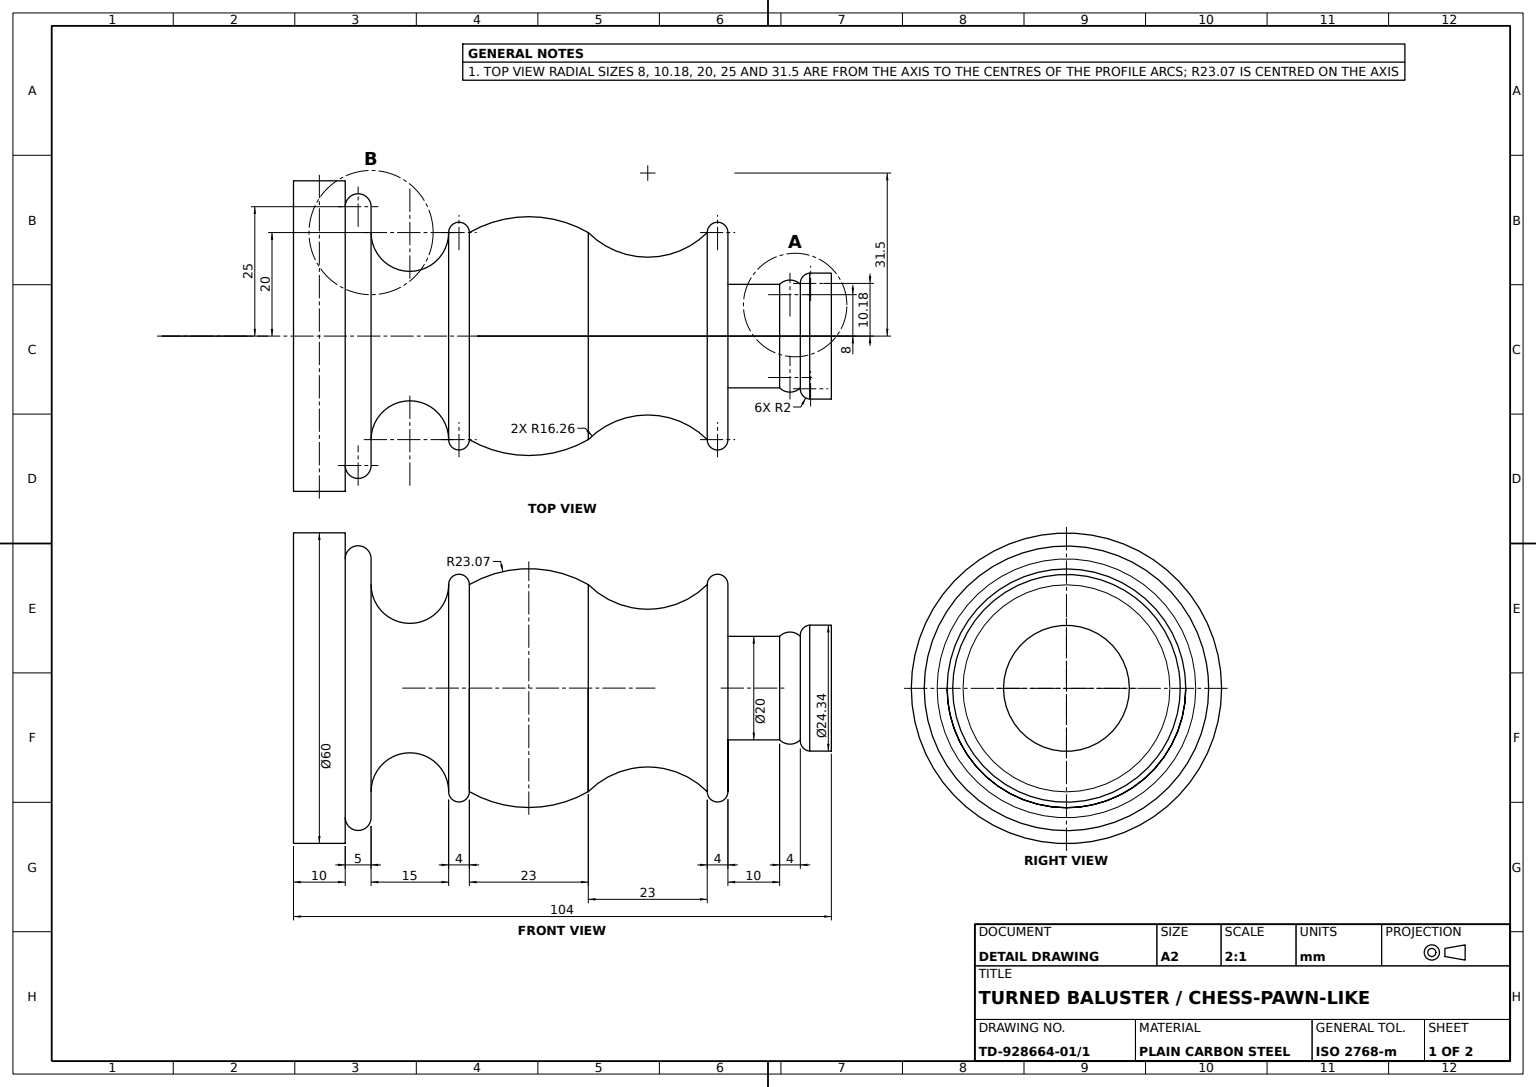
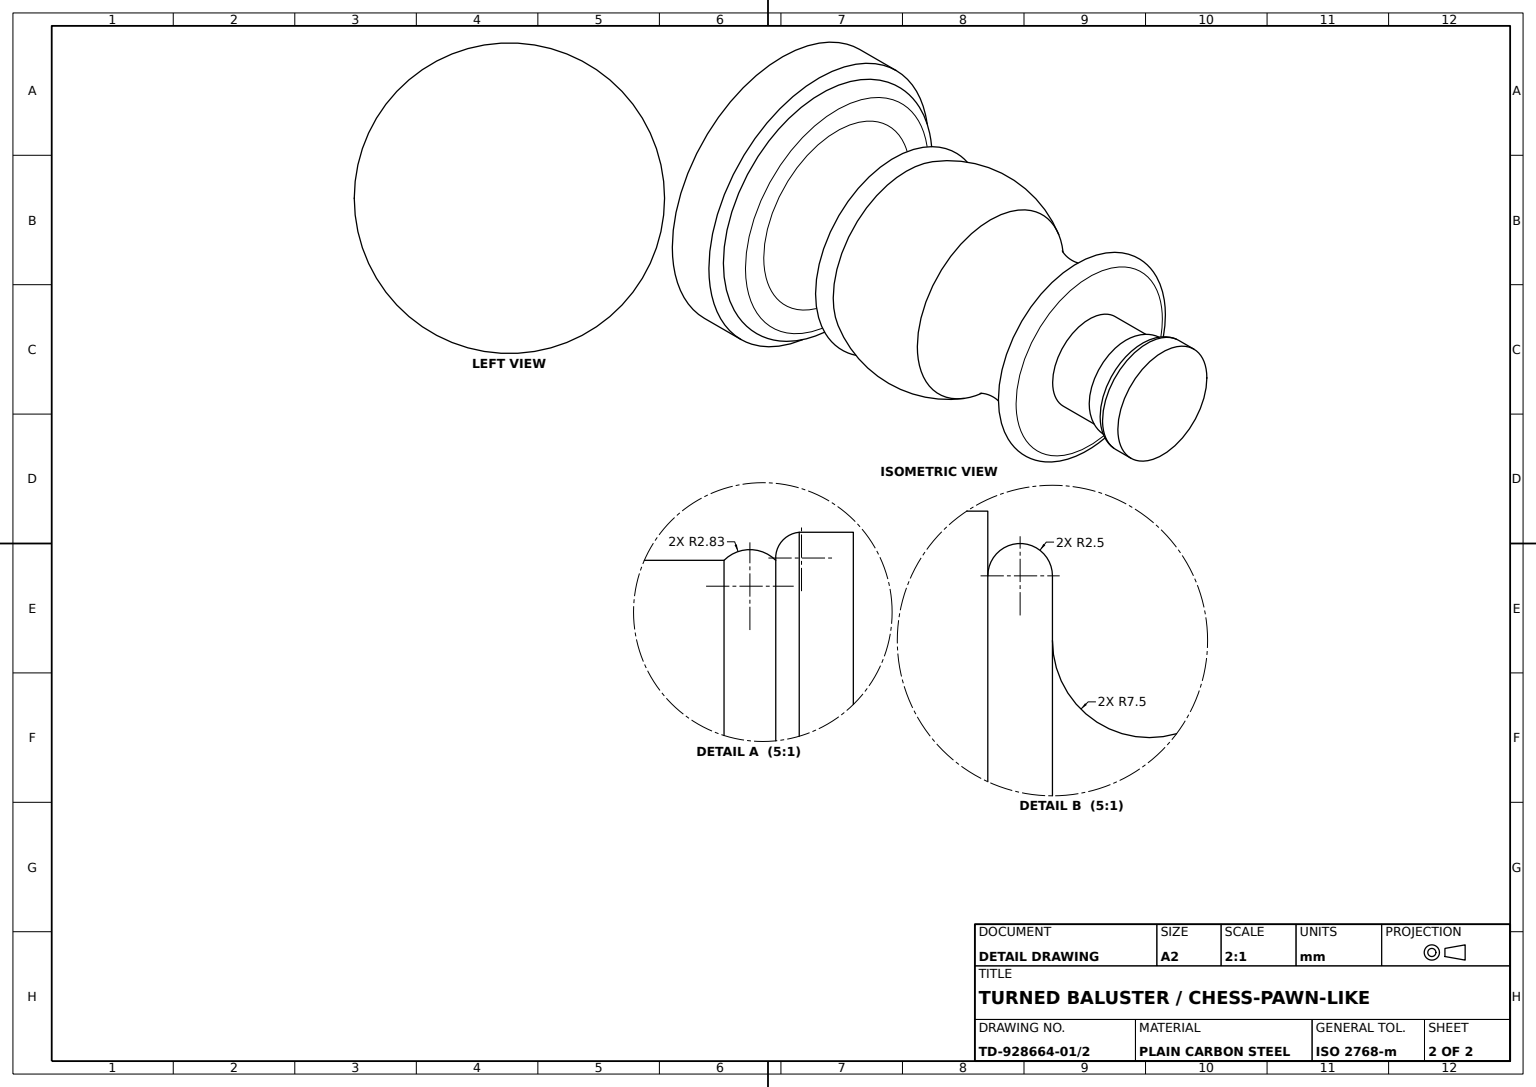
SolidWorks part; units mm, degrees
material "Plain Carbon Steel"
ref_plane "Front Plane" through (0, 0, 0) normal (0, 0, 1) x (1, 0, 0)
ref_plane "Top Plane" through (0, 0, 0) normal (0, 1, 0) x (1, 0, 0)
ref_plane "Right Plane" through (0, 0, 0) normal (1, 0, 0) x (0, 0, -1)
sketch "Baluster Half Profile" plane through (0, 0, 0) normal (0, 0, 1) x (1, 0, 0)
  line L0 (0, 0) -> (0, 104) construction
  line L1 (0, 0) -> (30, 0)
  line L2 (30, 0) -> (30, 10)
  line L3 (30, 10) -> (25, 10)
  line L4 (20, 30) -> (20, 15) construction
  line L5 (20, 15) -> (25, 15)
  line L6 (10, 84) -> (10, 94)
  line L7 (20, 84) -> (10, 84)
  line L8 (20, 34) -> (20, 30) construction
  line L9 (0, 0) -> (0, 104)
  line L10 (10.353, 98) -> (10, 98)
  line L13 (0, 104) -> (12.1687, 104)
  line L14 (12.1687, 104) -> (12.1687, 99.8157)
  arc A0 (25, 10) -> (25, 15) centre (25, 12.5) ccw
  arc A2 (20, 30) -> (20, 15) centre (20, 22.5) ccw
  arc A3 (20, 30) -> (20, 34) centre (20, 32) ccw
  arc A4 (20, 84) -> (20, 80) centre (20, 82) cw
  arc A6 (20, 34) -> (20, 57) centre (0, 45.5) ccw
  arc A7 (20, 57) -> (20, 80) centre (31.5, 68.5) cw
  arc A8 (10, 98) -> (10, 94) centre (8, 96) cw
  arc A9 (10.353, 98) -> (12.1687, 99.8157) centre (10.1765, 99.9922) ccw
  dimension "D3" = 7.5
  dimension "D2" = 2.5
  dimension "D4" = 2
  dimension "D5" = 23.0705
  dimension "D6" = 16.2635
  dimension "D7" = 2.8284
  dimension "D1" = 30
  dimension "D8" = 8
  dimension "D9" = 10
  dimension "D10" = 10.1765
  dimension "D11" = 12.1687
  dimension "D12" = 20
  dimension "D13" = 31.5
  dimension "D14" = 104
revolve "Baluster Body Revolve 360°" add sketch "Baluster Half Profile" angle 360 about L9
